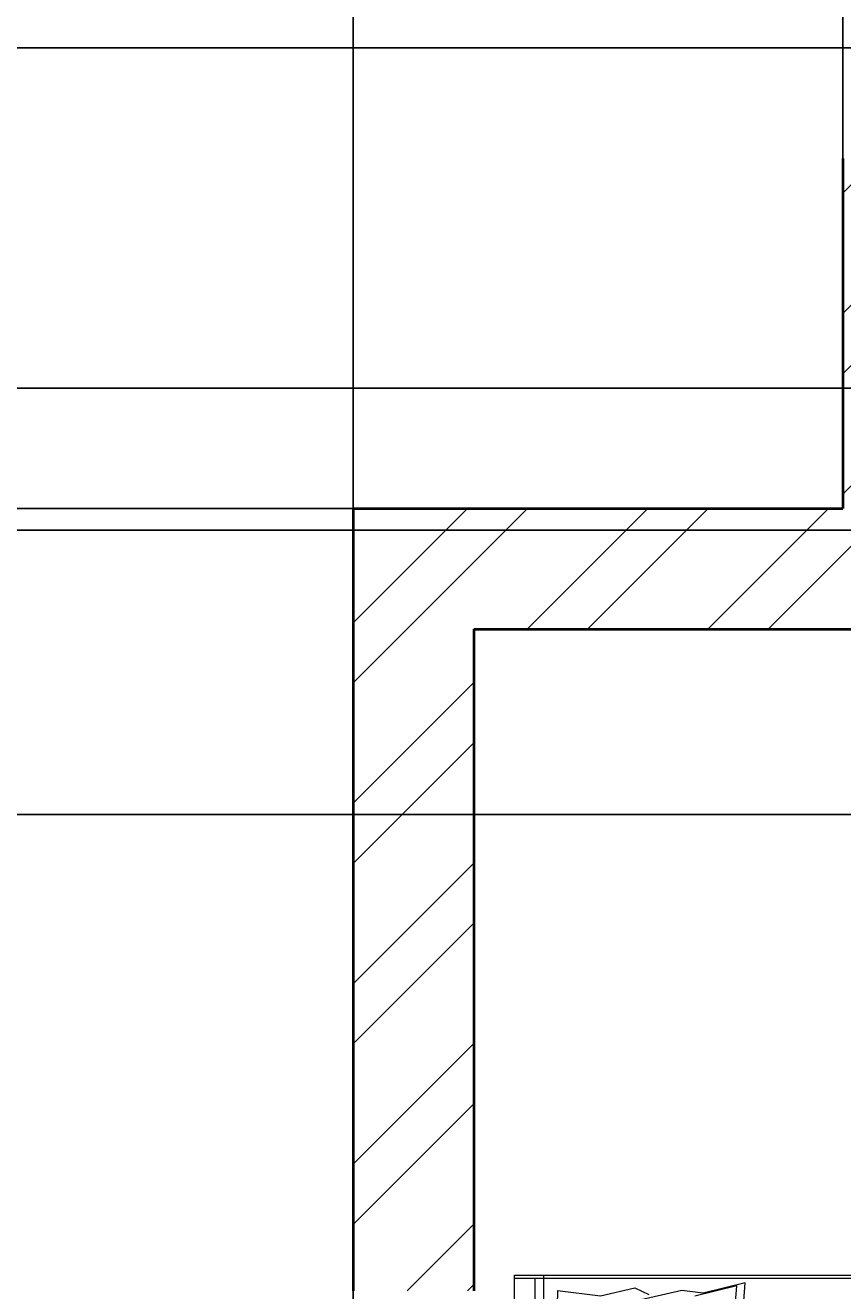
# Model space of a CAD drawing. Units: inches. Extents: x 1601 to 2297, y 1496 to 2631.
# Tile 10 of 57: x 1662 to 1723, y 1973 to 2067. Entities that reach past the tile are written whole.
import ezdxf

# ---------------------------------------------------------------- set-up
doc = ezdxf.new("R2010")
doc.units = ezdxf.units.IN
for name, color, linetype, lineweight in [('A-ANNO-DIMS', 2, 'Continuous', 18), ('A-FURN', 8, 'Continuous', 18), ('A-WALL', 7, 'Continuous', 40), ('A-WALL-PATT', 215, 'Continuous', 13)]:
    doc.layers.add(name, color=color, linetype=linetype, lineweight=lineweight)
doc.styles.get("Standard").update_dxf_attribs({"font": 'arial.ttf'})
doc.dimstyles.get("Standard").update_dxf_attribs({"dimtxt": 0.18, "dimasz": 0.18, "dimexe": 0.18, "dimexo": 0.0625, "dimgap": 0.09, "dimtad": 0, "dimtih": 1, "dimtoh": 1, "dimdec": 4, "dimzin": 0, "dimdsep": 46, "dimtxsty": 'Standard', "dimcen": 0.09, "dimadec": 0, "dimazin": 0, "dimtfac": 1, "dimtdec": 4, "dimtofl": 0, "dimtmove": 0, "dimatfit": 3, "dimfxl": 1, "dimtolj": 1, "dimtzin": 0, "dimarcsym": 0})

# ---------------------------------------------------------------- blocks, each defined once
blk = doc.blocks.new('BED-DOUBLE')
for p, q in [((0, 51.494), (0.639, 51.493)), ((0, 3.475), (0, 51.494)), ((0, 51.494), (0.639, 51.493)), ((0, 3.475), (0, 51.494)), ((0, 51.265), (26.61, 51.265)), ((0, 51.265), (26.61, 51.265)), ((0, 51.265), (26.61, 51.265)), ((0, 51.265), (26.61, 51.265)), ((0.639, 51.494), (27.249, 51.494)), ((0.639, 51.494), (27.249, 51.494)), ((0.639, 51.493), (27.249, 51.493)), ((0.639, 51.493), (27.249, 51.493)), ((1.533, 3.475), (1.533, 51.265)), ((1.533, 3.475), (1.533, 51.265)), ((1.533, 3.475), (1.533, 51.265)), ((1.533, 3.475), (1.533, 51.265)), ((2.173, 3.703), (2.173, 51.494)), ((2.173, 3.703), (2.173, 51.494)), ((2.173, 3.703), (2.173, 51.493)), ((2.173, 3.703), (2.173, 51.493)), ((3.196, 50.34), (3.099, 44.938)), ((3.196, 50.34), (3.099, 44.938)), ((3.196, 50.34), (3.099, 44.938)), ((3.196, 50.34), (3.099, 44.938)), ((3.196, 50.34), (6.407, 49.961)), ((3.196, 50.34), (6.407, 49.961)), ((3.196, 50.34), (6.407, 49.961)), ((3.196, 50.34), (6.407, 49.961)), ((6.407, 49.961), (8.977, 50.557)), ((6.407, 49.961), (8.977, 50.557)), ((6.407, 49.961), (8.977, 50.556)), ((6.407, 49.961), (8.977, 50.556)), ((12.468, 50.34), (8.896, 49.538)), ((12.468, 50.34), (8.896, 49.537)), ((12.468, 50.34), (8.896, 49.538)), ((12.468, 50.34), (8.896, 49.537)), ((8.977, 50.557), (10.024, 50.043)), ((8.977, 50.557), (10.024, 50.043)), ((8.977, 50.556), (10.024, 50.042)), ((8.977, 50.556), (10.024, 50.042)), ((14.073, 50.151), (12.468, 50.34)), ((14.073, 50.151), (12.468, 50.34)), ((14.073, 50.151), (12.468, 50.34)), ((14.073, 50.151), (12.468, 50.34)), ((16.573, 50.698), (13.434, 49.923)), ((16.573, 50.698), (13.434, 49.922)), ((16.573, 50.698), (13.434, 49.923)), ((16.573, 50.698), (13.434, 49.922)), ((17.212, 50.926), (14.073, 50.151)), ((17.212, 50.926), (14.073, 50.151)), ((17.212, 50.926), (14.073, 50.151)), ((17.212, 50.926), (14.073, 50.151)), ((16.169, 45.566), (16.573, 50.698)), ((16.169, 45.566), (16.573, 50.698)), ((16.169, 45.566), (16.573, 50.698)), ((16.169, 45.566), (16.573, 50.698)), ((16.808, 45.795), (17.212, 50.926)), ((16.808, 45.794), (17.212, 50.926)), ((16.808, 45.795), (17.212, 50.926)), ((16.808, 45.794), (17.212, 50.926))]:
    blk.add_line(p, q)
blk = doc.blocks.new('*D30')
at = {"layer": 'A-ANNO-DIMS', "color": 0, "lineweight": -2, "transparency": 16777216}
for p, q in [((1685.975, 2031.325), (1637.307, 2031.325)), ((1637.487, 2031.145), (1637.487, 1833.507)), ((1637.487, 1635.505), (1637.487, 1833.143)), ((1685.975, 1635.325), (1637.307, 1635.325))]:
    blk.add_line(p, q, dxfattribs=at)
at = {"layer": 'A-ANNO-DIMS', "color": 0, "transparency": 16777216}
for points in [[(1637.457, 2031.145), (1637.517, 2031.145), (1637.487, 2031.325)], [(1637.457, 1635.505), (1637.517, 1635.505), (1637.487, 1635.325)]]:
    blk.add_solid(points, dxfattribs=at)
at = {"layer": 'Defpoints', "color": 0, "transparency": 16777216}
for p in [(1637.487, 2031.325), (1686.037, 2031.325), (1686.037, 1635.325)]:
    blk.add_point(p, dxfattribs=at)
at = {"layer": 'A-ANNO-DIMS', "color": 0, "transparency": 16777216, "insert": (1637.487, 1833.325), "char_height": 0.18, "attachment_point": 5}
blk.add_mtext('\\A1;396', dxfattribs=at)
blk = doc.blocks.new('*D31')
at = {"layer": 'A-ANNO-DIMS', "color": 0, "lineweight": -2, "transparency": 16777216}
for p, q in [((1685.975, 2136.325), (1637.307, 2136.325)), ((1637.487, 2136.145), (1637.487, 2084.007)), ((1637.487, 2031.505), (1637.487, 2083.643)), ((1685.975, 2031.325), (1637.307, 2031.325))]:
    blk.add_line(p, q, dxfattribs=at)
at = {"layer": 'A-ANNO-DIMS', "color": 0, "transparency": 16777216}
for points in [[(1637.457, 2136.145), (1637.517, 2136.145), (1637.487, 2136.325)], [(1637.457, 2031.505), (1637.517, 2031.505), (1637.487, 2031.325)]]:
    blk.add_solid(points, dxfattribs=at)
at = {"layer": 'Defpoints', "color": 0, "transparency": 16777216}
for p in [(1637.487, 2136.325), (1686.037, 2136.325), (1686.037, 2031.325)]:
    blk.add_point(p, dxfattribs=at)
at = {"layer": 'A-ANNO-DIMS', "color": 0, "transparency": 16777216, "insert": (1637.487, 2083.825), "char_height": 0.18, "attachment_point": 5}
blk.add_mtext('\\A1;105', dxfattribs=at)
blk = doc.blocks.new('*D32')
at = {"layer": 'A-ANNO-DIMS', "color": 0, "lineweight": -2, "transparency": 16777216}
for p, q in [((1686.037, 2031.388), (1686.037, 2581.055)), ((1686.217, 2580.875), (1703.909, 2580.875)), ((1722.389, 2580.875), (1704.697, 2580.875)), ((1722.569, 2031.388), (1722.569, 2581.055))]:
    blk.add_line(p, q, dxfattribs=at)
at = {"layer": 'A-ANNO-DIMS', "color": 0, "transparency": 16777216}
for points in [[(1686.217, 2580.905), (1686.217, 2580.845), (1686.037, 2580.875)], [(1722.389, 2580.905), (1722.389, 2580.845), (1722.569, 2580.875)]]:
    blk.add_solid(points, dxfattribs=at)
at = {"layer": 'Defpoints', "color": 0, "transparency": 16777216}
for p in [(1722.569, 2580.875), (1686.037, 2031.325), (1722.569, 2031.325)]:
    blk.add_point(p, dxfattribs=at)
at = {"layer": 'A-ANNO-DIMS', "color": 0, "transparency": 16777216, "insert": (1704.303, 2580.875), "char_height": 0.18, "attachment_point": 5}
blk.add_mtext('\\A1;36.53', dxfattribs=at)
blk = doc.blocks.new('*D36')
at = {"layer": 'A-ANNO-DIMS', "color": 0, "lineweight": -2, "transparency": 16777216}
for p, q in [((1686.037, 1635.388), (1686.037, 2581.055)), ((1686.217, 2580.875), (1712.362, 2580.875)), ((1739.154, 2580.875), (1713.009, 2580.875)), ((1739.334, 1635.388), (1739.334, 2581.055))]:
    blk.add_line(p, q, dxfattribs=at)
at = {"layer": 'A-ANNO-DIMS', "color": 0, "transparency": 16777216}
for points in [[(1686.217, 2580.905), (1686.217, 2580.845), (1686.037, 2580.875)], [(1739.154, 2580.905), (1739.154, 2580.845), (1739.334, 2580.875)]]:
    blk.add_solid(points, dxfattribs=at)
at = {"layer": 'Defpoints', "color": 0, "transparency": 16777216}
for p in [(1739.334, 2580.875), (1686.037, 1635.325), (1739.334, 1635.325)]:
    blk.add_point(p, dxfattribs=at)
at = {"layer": 'A-ANNO-DIMS', "color": 0, "transparency": 16777216, "insert": (1712.685, 2580.875), "char_height": 0.18, "attachment_point": 5}
blk.add_mtext('\\A1;53.3', dxfattribs=at)
blk = doc.blocks.new('*D42')
at = {"layer": 'A-ANNO-DIMS', "color": 0, "lineweight": -2, "transparency": 16777216}
for p, q in [((2177.975, 2065.697), (1637.307, 2065.697)), ((1637.487, 2065.517), (1637.487, 2047.878)), ((1637.487, 2029.877), (1637.487, 2047.515)), ((2177.975, 2029.697), (1637.307, 2029.697))]:
    blk.add_line(p, q, dxfattribs=at)
at = {"layer": 'A-ANNO-DIMS', "color": 0, "transparency": 16777216}
for points in [[(1637.457, 2065.517), (1637.517, 2065.517), (1637.487, 2065.697)], [(1637.457, 2029.877), (1637.517, 2029.877), (1637.487, 2029.697)]]:
    blk.add_solid(points, dxfattribs=at)
at = {"layer": 'Defpoints', "color": 0, "transparency": 16777216}
for p in [(1637.487, 2065.697), (2178.037, 2065.697), (2178.037, 2029.697)]:
    blk.add_point(p, dxfattribs=at)
at = {"layer": 'A-ANNO-DIMS', "color": 0, "transparency": 16777216, "insert": (1637.487, 2047.697), "char_height": 0.18, "attachment_point": 5}
blk.add_mtext('\\A1;36', dxfattribs=at)
blk = doc.blocks.new('*D45')
at = {"layer": 'A-ANNO-DIMS', "color": 0, "lineweight": -2, "transparency": 16777216}
for p, q in [((1958.975, 2040.303), (1637.307, 2040.303)), ((1637.487, 2040.123), (1637.487, 2024.571)), ((1637.487, 2008.656), (1637.487, 2024.207)), ((1958.975, 2008.476), (1637.307, 2008.476))]:
    blk.add_line(p, q, dxfattribs=at)
at = {"layer": 'A-ANNO-DIMS', "color": 0, "transparency": 16777216}
for points in [[(1637.457, 2040.123), (1637.517, 2040.123), (1637.487, 2040.303)], [(1637.457, 2008.656), (1637.517, 2008.656), (1637.487, 2008.476)]]:
    blk.add_solid(points, dxfattribs=at)
at = {"layer": 'Defpoints', "color": 0, "transparency": 16777216}
for p in [(1637.487, 2040.303), (1959.037, 2040.303), (1959.037, 2008.476)]:
    blk.add_point(p, dxfattribs=at)
at = {"layer": 'A-ANNO-DIMS', "color": 0, "transparency": 16777216, "insert": (1637.487, 2024.389), "char_height": 0.18, "attachment_point": 5}
blk.add_mtext('\\A1;31.83', dxfattribs=at)

msp = doc.modelspace()

# ---------------------------------------------------------------- hatches: boundary and pattern name
at = {"layer": 'A-WALL-PATT'}
h = msp.add_hatch(dxfattribs=at)
h.set_pattern_fill('ANSI32', color=256)
h.paths.add_polyline_path([(2230.5373, 1861.8254), (2182.5373, 1861.8254), (2182.5373, 1885.3637), (2178.0373, 1885.3637), (2178.0373, 1861.8254), (2166.0373, 1861.8254), (2134.5373, 1861.8254), (2130.0373, 1861.8254), (2130.0373, 1841.4682), (2126.8833, 1841.4682), (2126.8833, 1836.9682), (2130.0373, 1836.9682), (2130.0373, 1822.7302), (2134.5373, 1822.7302), (2134.5373, 1857.3254), (2166.0373, 1857.3254), (2226.0373, 1857.3254), (2226.0373, 1846.1155), (2230.5373, 1846.1155)])
h.paths.add_polyline_path([(2226.0373, 1797.3254), (2134.5373, 1797.3254), (2134.5373, 1800.6636), (2132.2873, 1800.6636), (2130.0373, 1800.6636), (2130.0373, 1797.3254), (2130.0373, 1792.8254), (2167.7264, 1792.8254), (2226.0373, 1792.8254)])
h.paths.add_polyline_path([(2230.5373, 1822.1155), (2226.0373, 1822.1155), (2226.0373, 1760.8563), (2230.5373, 1760.8563)])
h.paths.add_polyline_path([(2230.5373, 1700.8563), (2226.0373, 1700.8563), (2226.0373, 1644.3254), (2140.2517, 1644.3254), (2140.2517, 1635.3254), (2230.5373, 1635.3254)])
h.paths.add_polyline_path([(2080.2517, 1639.8254), (2080.2517, 1644.3254), (2035.5373, 1644.3254), (2035.5373, 1792.8254), (2094.0373, 1792.8254), (2094.0373, 1797.3254), (2094.0373, 1836.9682), (2097.1057, 1836.9682), (2097.1057, 1839.2182), (2097.1057, 1841.4682), (2094.0373, 1841.4682), (2094.0373, 1862.2276), (2089.5373, 1862.2276), (2089.5373, 1797.3254), (2035.5373, 1797.3254), (2035.5373, 1857.3254), (2035.5373, 1885.0916), (2031.0373, 1885.0916), (2031.0373, 1710.3254), (2012.329, 1710.3254), (2012.329, 1701.3254), (2031.0373, 1701.3254), (2031.0373, 1644.3254), (2031.0373, 1635.3254), (2080.2517, 1635.3254)])
h.paths.add_polyline_path([(1836.0373, 1653.2033), (1842.6171, 1653.2033), (1842.6171, 1657.7033), (1842.6171, 1662.2033), (1831.5373, 1662.2033), (1831.5373, 1764.2033), (1835.3881, 1764.2033), (1835.3881, 1766.4533), (1835.3881, 1768.7033), (1831.5373, 1768.7033), (1827.0373, 1768.7033), (1827.0373, 1662.2033), (1827.0373, 1635.3254), (1836.0373, 1635.3254)])
h.paths.add_polyline_path([(1893.0373, 1701.3254), (1907.193, 1701.3254), (1907.193, 1705.8254), (1907.193, 1710.3254), (1893.0373, 1710.3254), (1893.0373, 1819.8254), (1882.6444, 1819.8254), (1882.6444, 1817.5754), (1882.6444, 1815.3254), (1888.5373, 1815.3254), (1888.5373, 1662.2033), (1884.0373, 1662.2033), (1866.6171, 1662.2033), (1866.6171, 1653.2033), (1882.391, 1653.2033), (1884.0373, 1653.2033), (1884.0373, 1635.3254), (1893.0373, 1635.3254)])
h.paths.add_polyline_path([(1739.3335, 1639.8254), (1739.3335, 1644.3254), (1695.0373, 1644.3254), (1695.0373, 1702.0135), (1690.5373, 1702.0135), (1686.0373, 1702.0135), (1686.0373, 1635.3254), (1739.3335, 1635.3254)])
h.paths.add_polyline_path([(1827.0373, 1644.3254), (1799.3335, 1644.3254), (1799.3335, 1635.3254), (1827.0373, 1635.3254)])
h.paths.add_polyline_path([(1695.0373, 1815.3254), (1849.2759, 1815.3254), (1849.2759, 1819.8254), (1807.5373, 1819.8254), (1807.5373, 1879.8254), (1851.1533, 1879.8254), (1851.1533, 1882.0754), (1851.1533, 1884.3254), (1799.3405, 1884.3254), (1799.3405, 1882.0754), (1799.3405, 1879.8254), (1803.0373, 1879.8254), (1803.0373, 1819.8254), (1695.0373, 1819.8254), (1695.0373, 1835.0458), (1690.5373, 1835.0458), (1686.0373, 1835.0458), (1686.0373, 1766.1753), (1695.0373, 1766.1753)])
h.paths.add_polyline_path([(1775.8157, 1884.3254), (1695.0373, 1884.3254), (1695.0373, 1912.9526), (1690.5373, 1912.9526), (1686.0373, 1912.9526), (1686.0373, 1859.0458), (1695.0373, 1859.0458), (1695.0373, 1879.8254), (1775.8157, 1879.8254)])
h.paths.add_polyline_path([(1893.0373, 2031.3254), (1731.5687, 2031.3254), (1731.5687, 2057.4352), (1722.5687, 2057.4352), (1722.5687, 2031.3254), (1686.0373, 2031.3254), (1686.0373, 1972.9526), (1695.0373, 1972.9526), (1695.0373, 2022.3254), (1888.5373, 2022.3254), (1888.5373, 1884.3254), (1883.4996, 1884.3254), (1883.4996, 1879.8254), (1893.0373, 1879.8254), (1893.0373, 1974.3254), (1976.6199, 1974.3254), (1976.6199, 1978.8254), (1968.0373, 1978.8254), (1968.0373, 1983.3254), (1968.0373, 2008.4756), (1963.5373, 2008.4756), (1959.0373, 2008.4756), (1959.0373, 1983.3254), (1893.0373, 1983.3254)])
h.paths.add_polyline_path([(2230.5373, 2140.4745), (2226.0373, 2140.4745), (2226.0373, 2094.3254), (2040.0373, 2094.3254), (2040.0373, 2085.3254), (2178.0373, 2085.3254), (2178.0373, 2065.6965), (2182.5373, 2065.6965), (2182.5373, 2085.3254), (2226.0373, 2085.3254), (2226.0373, 1986.3254), (2211.2679, 1986.3254), (2211.2679, 1981.8254), (2230.5373, 1981.8254)])
h.paths.add_polyline_path([(2187.6292, 1986.3254), (2182.5373, 1986.3254), (2182.5373, 2029.6965), (2178.0373, 2029.6965), (2178.0373, 1986.3254), (2099.05, 1986.3254), (2099.05, 1981.8254), (2178.0373, 1981.8254), (2178.0373, 1969.3637), (2182.5373, 1969.3637), (2182.5373, 1981.8254), (2187.6292, 1981.8254), (2187.6292, 1984.0754)])
h.paths.add_polyline_path([(1807.1169, 1573.5395), (2055.0405, 1573.5395), (2055.0405, 1610.6322), (1807.1169, 1610.6322)], flags=9)
h.paths.add_polyline_path([(1841.1631, 1712.7967), (1870.3957, 1712.7967), (1870.3957, 1731.454), (1841.1631, 1731.454)], flags=9)
h.paths.add_polyline_path([(2144.3862, 1772.185), (2191.0233, 1772.185), (2191.0233, 1790.8423), (2144.3862, 1790.8423)], flags=9)
h.paths.add_polyline_path([(2143.0128, 1827.3312), (2177.9958, 1827.3312), (2177.9958, 1845.9886), (2143.0128, 1845.9886)], flags=25)
h.paths.add_polyline_path([(2041.2439, 1833.5691), (2070.8516, 1833.5691), (2070.8516, 1852.2264), (2041.2439, 1852.2264)], flags=25)
h.paths.add_polyline_path([(2097.2791, 1947.0598), (2134.2061, 1947.0598), (2134.2061, 1965.7171), (2097.2791, 1965.7171)], flags=9)
h.paths.add_polyline_path([(2214.995, 1904.3124), (2214.995, 1942.2899), (2196.3376, 1942.2899), (2196.3376, 1904.3124)], flags=9)
h.paths.add_polyline_path([(2186.6284, 2043.8031), (2219.7935, 2043.8031), (2219.7935, 2062.4605), (2186.6284, 2062.4605)], flags=25)
h.paths.add_polyline_path([(2064.0877, 2031.616), (2097.4949, 2031.616), (2097.4949, 2050.2734), (2064.0877, 2050.2734)], flags=25)
h.paths.add_polyline_path([(1973.1349, 1986.0688), (2008.4009, 1986.0688), (2008.4009, 2004.7261), (1973.1349, 2004.7261)], flags=9)
h.paths.add_polyline_path([(1976.3676, 2106.9635), (2005.7469, 2106.9635), (2005.7469, 2125.6209), (1976.3676, 2125.6209)], flags=9)
h.paths.add_polyline_path([(1991.7852, 2180.4863), (2027.0513, 2180.4863), (2027.0513, 2199.1437), (1991.7852, 2199.1437)], flags=9)
h.paths.add_polyline_path([(2106.1801, 2187.9359), (2152.2101, 2187.9359), (2152.2101, 2206.5932), (2106.1801, 2206.5932)], flags=9)
h.paths.add_polyline_path([(2148.6686, 2262.2542), (2182.318, 2262.2542), (2182.318, 2280.9115), (2148.6686, 2280.9115)], flags=9)
h.paths.add_polyline_path([(2041.6327, 2252.8147), (2071.2405, 2252.8147), (2071.2405, 2271.4721), (2041.6327, 2271.4721)], flags=9)
h.paths.add_polyline_path([(2063.9734, 2375.4265), (2100.9004, 2375.4265), (2100.9004, 2394.0839), (2063.9734, 2394.0839)], flags=9)
h.paths.add_polyline_path([(2216.4955, 2330.9748), (2216.4955, 2370.2654), (2197.8381, 2370.2654), (2197.8381, 2330.9748)], flags=9)
h.paths.add_polyline_path([(2179.1416, 2485.8687), (2212.3067, 2485.8687), (2212.3067, 2504.5261), (2179.1416, 2504.5261)], flags=9)
h.paths.add_polyline_path([(2078.7442, 2471.1516), (2112.1514, 2471.1516), (2112.1514, 2489.809), (2078.7442, 2489.809)], flags=9)
h.paths.add_polyline_path([(1915.9631, 2329.4668), (1952.8902, 2329.4668), (1952.8902, 2348.1241), (1915.9631, 2348.1241)], flags=9)
h.paths.add_polyline_path([(1904.3189, 2499.6709), (1940.4512, 2499.6709), (1940.4512, 2518.3282), (1904.3189, 2518.3282)], flags=9)
h.paths.add_polyline_path([(1892.3665, 2100.4595), (1925.6374, 2100.4595), (1925.6374, 2119.1169), (1892.3665, 2119.1169)], flags=9)
h.paths.add_polyline_path([(1909.2984, 1805.9631), (1946.2254, 1805.9631), (1946.2254, 1824.6205), (1909.2984, 1824.6205)], flags=9)
h.paths.add_polyline_path([(1934.6056, 1658.616), (1970.738, 1658.616), (1970.738, 1677.2733), (1934.6056, 1677.2733)], flags=9)
h.paths.add_polyline_path([(1711.2052, 1789.8902), (1750.0456, 1789.8902), (1750.0456, 1808.5476), (1711.2052, 1808.5476)], flags=25)
h.paths.add_polyline_path([(1742.7874, 1854.6743), (1771.9449, 1854.6743), (1771.9449, 1873.3317), (1742.7874, 1873.3317)], flags=25)
h.paths.add_polyline_path([(1807.3592, 1997.7912), (1850.1116, 1997.7912), (1850.1116, 2016.4486), (1807.3592, 2016.4486)], flags=25)
h.paths.add_polyline_path([(1717.4579, 2237.7844), (1760.2103, 2237.7844), (1760.2103, 2256.4417), (1717.4579, 2256.4417)], flags=9)
h.paths.add_polyline_path([(1780.9285, 2324.0623), (1810.086, 2324.0623), (1810.086, 2342.7197), (1780.9285, 2342.7197)], flags=9)
h.paths.add_polyline_path([(1837.696, 2449.2024), (1866.9286, 2449.2024), (1866.9286, 2467.8598), (1837.696, 2467.8598)], flags=9)
h.paths.add_polyline_path([(1712.7752, 2484.9404), (1751.6156, 2484.9404), (1751.6156, 2503.5977), (1712.7752, 2503.5977)], flags=9)

# ---------------------------------------------------------------- linework, layer by layer
at = {"layer": 'A-WALL'}
for p, q in [((1722.5687, 2057.4352), (1722.5687, 2031.3254)), ((1686.0373, 2031.3254), (1722.5687, 2031.3254)), ((1686.0373, 2031.3254), (1686.0373, 1972.9526)), ((1695.0373, 2022.3254), (1888.5373, 2022.3254)), ((1695.0373, 2022.3254), (1695.0373, 1972.9526))]:
    msp.add_line(p, q, dxfattribs=at)

# ---------------------------------------------------------------- block references
at = {"layer": 'A-FURN'}
msp.add_blockref('BED-DOUBLE', (1698.0921, 1922.6184), dxfattribs=at)

# ---------------------------------------------------------------- dimensions: what is measured, and where the dimension line sits
at = {"layer": 'A-ANNO-DIMS'}
for base, p1, p2, override, picture, middle in [((1722.5687, 2580.8754), (1686.0373, 2031.3254), (1722.5687, 2031.3254), {"dimdec": 2, "dimlfac": 1, "dimrnd": 0, "dimzin": 0, "dimdsep": 46, "dimlunit": 2}, '*D32', (1704.303, 2580.8754)), ((1739.3335, 2580.8754), (1686.0373, 1635.3254), (1739.3335, 1635.3254), {"dimdec": 1, "dimlfac": 1, "dimrnd": 0, "dimzin": 0, "dimdsep": 46, "dimlunit": 2}, '*D36', (1712.6854, 2580.8754))]:
    dim = msp.add_linear_dim(base=base, p1=p1, p2=p2, dimstyle='Standard', override=override, dxfattribs=at)
    dim.commit()
    dim.dimension.update_dxf_attribs({"geometry": picture, "text_midpoint": middle})
for base, p1, p2, override, picture, middle in [((1637.4873, 2136.3254), (1686.0373, 2031.3254), (1686.0373, 2136.3254), {"dimdec": 0, "dimlfac": 1, "dimrnd": 0, "dimzin": 0, "dimdsep": 46, "dimlunit": 2}, '*D31', (1637.4873, 2083.8254)), ((1637.4873, 2065.6965), (2178.0373, 2029.6965), (2178.0373, 2065.6965), {"dimdec": 0, "dimlfac": 1, "dimrnd": 0, "dimzin": 0, "dimdsep": 46, "dimlunit": 2}, '*D42', (1637.4873, 2047.6965)), ((1637.4873, 2040.3029), (1959.0373, 2008.4756), (1959.0373, 2040.3029), {"dimdec": 2, "dimlfac": 1, "dimrnd": 0, "dimzin": 0, "dimdsep": 46, "dimlunit": 2}, '*D45', (1637.4873, 2024.3893)), ((1637.4873, 2031.3254), (1686.0373, 1635.3254), (1686.0373, 2031.3254), {"dimdec": 0, "dimlfac": 1, "dimrnd": 0, "dimzin": 0, "dimdsep": 46, "dimlunit": 2}, '*D30', (1637.4873, 1833.3254))]:
    dim = msp.add_linear_dim(base=base, p1=p1, p2=p2, angle=90, dimstyle='Standard', override=override, dxfattribs=at)
    dim.commit()
    dim.dimension.update_dxf_attribs({"geometry": picture, "text_midpoint": middle})

doc.saveas('drawing.dxf')
